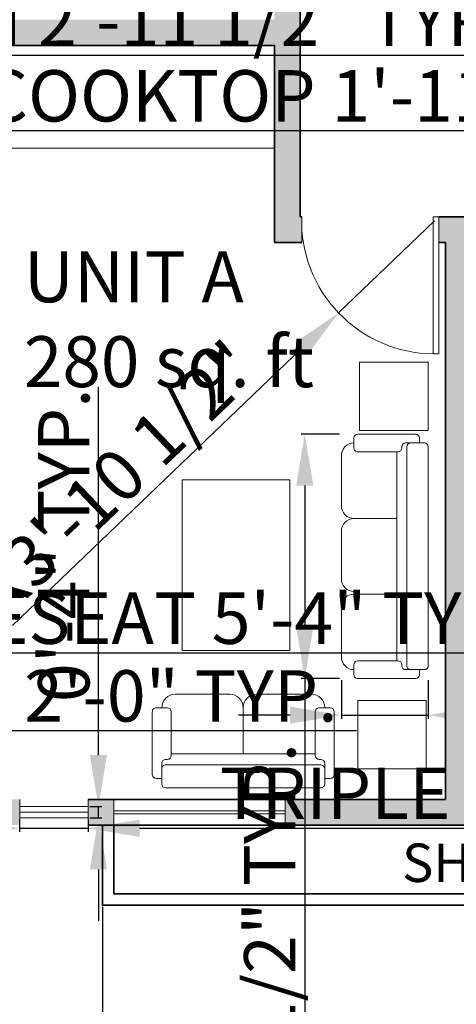
# Model space of a CAD drawing. Units: inches. Extents: x 2043 to 3177, y 1429 to 2563.
# Tile 6 of 14: x 2453 to 2607, y 1608 to 1952. Entities that reach past the tile are written whole.
import ezdxf

# ---------------------------------------------------------------- set-up
doc = ezdxf.new("R2010")
doc.units = ezdxf.units.IN
for name, color, linetype, lineweight in [('A-ANNO-DIMS', 2, 'Continuous', 13), ('A-AREA-IDEN', 7, 'Continuous', 18), ('A-DOOR', 3, 'Continuous', 18), ('A-FLOR-CASE', 8, 'Continuous', 18), ('A-FURN', 8, 'Continuous', 18), ('A-GLAZ', 4, 'Continuous', 18), ('A-WALL', 7, 'Continuous', 35)]:
    doc.layers.add(name, color=color, linetype=linetype, lineweight=lineweight)
doc.layers.add('A-WALL-PATT', color=251, linetype='Continuous', lineweight=13, true_color=0x636466)
doc.styles.get("Standard").update_dxf_attribs({"font": 'arial.ttf'})
doc.dimstyles.new('ISO-25', dxfattribs={"dimtxt": 18, "dimasz": 18, "dimexe": 1.25, "dimexo": 0.625, "dimtad": 1, "dimlunit": 3, "dimtxsty": 'Standard', "dimcen": 2.5, "dimadec": 0, "dimazin": 0, "dimtfac": 1, "dimtmove": 0, "dimatfit": 3, "dimfxl": 1, "dimarcsym": 0})

# ---------------------------------------------------------------- blocks, each defined once
blk = doc.blocks.new('A$C115861F8')
for p, q in [((0.0679, 0.6401), (0.0679, 0.6013)), ((1.7846, 0.6692), (0.097, 0.6692)), ((1.8136, 0.6401), (1.8136, 0.6013)), ((0, 0.5722), (0, 0.1261)), ((0.0679, 0.6013), (0.0291, 0.6013)), ((0.0679, 0.5334), (0.0679, 0.6013)), ((0.0679, 0.4946), (0.0679, 0.5431)), ((1.8136, 0.6013), (1.8524, 0.6013)), ((1.8136, 0.5334), (1.8136, 0.6013)), ((1.8136, 0.4946), (1.8136, 0.5431)), ((1.8815, 0.5722), (1.8815, 0.1261)), ((1.7846, 0.5043), (0.097, 0.5043)), ((0.1067, 0.4655), (0.097, 0.4655)), ((1.7749, 0.4655), (1.7846, 0.4655)), ((0.1358, 0.1261), (0.1358, 0.4364)), ((1.7458, 0.4267), (0.1358, 0.4267)), ((0.6498, 0.097), (0.6498, 0.4267)), ((1.2317, 0.097), (1.2317, 0.4267)), ((1.7458, 0.1261), (1.7458, 0.4364)), ((0.0291, 0.097), (0.1067, 0.097)), ((1.8524, 0.097), (1.7749, 0.097)), ((0.1649, 0), (0.5528, 0)), ((1.1347, 0), (0.7468, 0)), ((1.3287, 0), (1.7167, 0))]:
    blk.add_line(p, q)
for centre, radius, start, end in [((0.097, 0.6401), 0.0291, 90, 180), ((1.7846, 0.6401), 0.0291, 0, 90), ((0.0291, 0.5722), 0.0291, 90, 180), ((0.097, 0.5334), 0.0291, 180, 270), ((1.7846, 0.5334), 0.0291, 270, 0), ((1.8524, 0.5722), 0.0291, 0, 90), ((0.097, 0.4946), 0.0291, 180, 270), ((0.1067, 0.4364), 0.0291, 0, 90), ((1.7749, 0.4364), 0.0291, 90, 180), ((1.7846, 0.4946), 0.0291, 270, 0), ((0.0291, 0.1261), 0.0291, 180, 270), ((0.1649, 0.097), 0.097, 180, 270), ((0.1067, 0.1261), 0.0291, 270, 0), ((0.5528, 0.097), 0.097, 270, 0), ((0.7468, 0.097), 0.097, 180, 270), ((1.1147, 0.097), 0.097, 270, 0), ((1.3287, 0.097), 0.097, 180, 270), ((1.7167, 0.097), 0.097, 270, 0), ((1.7749, 0.1261), 0.0291, 180, 270), ((1.8524, 0.1261), 0.0291, 270, 0)]:
    blk.add_arc(centre, radius, start, end)
blk = doc.blocks.new('A$C02A636C4')
for p, q in [((0.0679, 0.6401), (0.0679, 0.6013)), ((1.2026, 0.6692), (0.097, 0.6692)), ((1.2317, 0.6401), (1.2317, 0.6013)), ((0, 0.5722), (0, 0.1261)), ((0.0679, 0.6013), (0.0291, 0.6013)), ((0.0679, 0.5334), (0.0679, 0.6013)), ((1.2317, 0.6013), (1.2705, 0.6013)), ((1.2317, 0.5334), (1.2317, 0.6013)), ((1.2996, 0.5722), (1.2996, 0.1261)), ((0.0679, 0.4946), (0.0679, 0.5431)), ((1.2026, 0.5043), (0.097, 0.5043)), ((1.2317, 0.4946), (1.2317, 0.5431)), ((0.1067, 0.4655), (0.097, 0.4655)), ((0.1358, 0.1261), (0.1358, 0.4364)), ((1.1638, 0.4267), (0.1358, 0.4267)), ((0.6498, 0.097), (0.6498, 0.4267)), ((1.1638, 0.1261), (1.1638, 0.4364)), ((1.1929, 0.4655), (1.2026, 0.4655)), ((0.0291, 0.097), (0.1067, 0.097)), ((1.2705, 0.097), (1.1929, 0.097)), ((0.1649, 0), (0.5528, 0)), ((0.7468, 0), (1.1347, 0))]:
    blk.add_line(p, q)
for centre, radius, start, end in [((0.097, 0.6401), 0.0291, 90, 180), ((1.2026, 0.6401), 0.0291, 0, 90), ((0.0291, 0.5722), 0.0291, 90, 180), ((1.2705, 0.5722), 0.0291, 0, 90), ((0.097, 0.5334), 0.0291, 180, 270), ((0.097, 0.4946), 0.0291, 180, 270), ((1.2026, 0.5334), 0.0291, 270, 0), ((1.2026, 0.4946), 0.0291, 270, 0), ((0.1067, 0.4364), 0.0291, 0, 90), ((1.1929, 0.4364), 0.0291, 90, 180), ((0.0291, 0.1261), 0.0291, 180, 270), ((0.1649, 0.097), 0.097, 180, 270), ((0.1067, 0.1261), 0.0291, 270, 0), ((0.5528, 0.097), 0.097, 270, 0), ((0.7468, 0.097), 0.097, 180, 270), ((1.1347, 0.097), 0.097, 270, 0), ((1.1929, 0.1261), 0.0291, 180, 270), ((1.2705, 0.1261), 0.0291, 270, 0)]:
    blk.add_arc(centre, radius, start, end)
blk = doc.blocks.new('*D22')
at = {"layer": 'A-ANNO-DIMS', "color": 0, "lineweight": -2, "transparency": 16777216}
for p, q in [((2482.49, 1641.77), (2482.49, 1560.37)), ((2731.99, 1641.77), (2731.99, 1560.37)), ((2500.49, 1561.62), (2713.99, 1561.62))]:
    blk.add_line(p, q, dxfattribs=at)
at = {"layer": 'A-ANNO-DIMS', "color": 0, "transparency": 16777216}
for points in [[(2500.49, 1564.62), (2500.49, 1558.62), (2482.49, 1561.62)], [(2713.99, 1564.62), (2713.99, 1558.62), (2731.99, 1561.62)]]:
    blk.add_solid(points, dxfattribs=at)
at = {"layer": 'Defpoints', "color": 0, "transparency": 16777216}
for p in [(2482.49, 1642.39), (2731.99, 1642.39), (2731.99, 1561.62)]:
    blk.add_point(p, dxfattribs=at)
at = {"layer": 'A-ANNO-DIMS', "color": 0, "transparency": 16777216, "insert": (2607.24, 1571.44), "char_height": 18, "attachment_point": 5}
blk.add_mtext('25\'-0"', dxfattribs=at)
blk = doc.blocks.new('*D23')
at = {"layer": 'A-ANNO-DIMS', "color": 0, "lineweight": -2, "transparency": 16777216}
for p, q in [((2446.74, 1641.77), (2446.74, 1511.06)), ((2482.49, 1641.77), (2482.49, 1511.06)), ((2428.74, 1512.31), (2361.66, 1512.31)), ((2482.49, 1512.31), (2446.74, 1512.31)), ((2500.49, 1512.31), (2518.49, 1512.31))]:
    blk.add_line(p, q, dxfattribs=at)
at = {"layer": 'A-ANNO-DIMS', "color": 0, "transparency": 16777216}
for points in [[(2428.74, 1515.31), (2428.74, 1509.31), (2446.74, 1512.31)], [(2500.49, 1515.31), (2500.49, 1509.31), (2482.49, 1512.31)]]:
    blk.add_solid(points, dxfattribs=at)
at = {"layer": 'Defpoints', "color": 0, "transparency": 16777216}
for p in [(2446.74, 1642.39), (2482.49, 1642.39), (2446.74, 1512.31)]:
    blk.add_point(p, dxfattribs=at)
at = {"layer": 'A-ANNO-DIMS', "color": 0, "transparency": 16777216, "insert": (2386.2, 1522.13), "char_height": 18, "attachment_point": 5}
blk.add_mtext('3\'-0"', dxfattribs=at)
blk = doc.blocks.new('*D29')
at = {"layer": 'A-ANNO-DIMS', "color": 0, "lineweight": -2, "transparency": 16777216}
for p, q in [((2233.74, 1633.77), (2233.74, 1430.58)), ((2980.74, 1633.77), (2980.74, 1430.58)), ((2251.74, 1431.83), (2962.74, 1431.83))]:
    blk.add_line(p, q, dxfattribs=at)
at = {"layer": 'A-ANNO-DIMS', "color": 0, "transparency": 16777216}
for points in [[(2251.74, 1434.83), (2251.74, 1428.83), (2233.74, 1431.83)], [(2962.74, 1434.83), (2962.74, 1428.83), (2980.74, 1431.83)]]:
    blk.add_solid(points, dxfattribs=at)
at = {"layer": 'Defpoints', "color": 0, "transparency": 16777216}
for p in [(2233.74, 1634.39), (2980.74, 1634.39), (2980.74, 1431.83)]:
    blk.add_point(p, dxfattribs=at)
at = {"layer": 'A-ANNO-DIMS', "color": 0, "transparency": 16777216, "insert": (2607.24, 1441.64), "char_height": 18, "attachment_point": 5}
blk.add_mtext('75\'-0"', dxfattribs=at)
blk = doc.blocks.new('END-TABLE-24')
blk.add_lwpolyline([(24, 24), (24, 0), (0, 0), (0, 24)], close=True)
blk = doc.blocks.new('COFFEE-TABLE-RECT')
blk.add_lwpolyline([(0, 59.71), (37.81, 59.71), (37.81, 0), (0, 0)], close=True)
blk = doc.blocks.new('GLAZING-24-TRIPLE')
for p, q in [((24, 4), (0, 4)), ((24, 2), (0, 2)), ((24, 0), (0, 0))]:
    blk.add_line(p, q)
blk = doc.blocks.new('GLAZING-60')
for p, q in [((0, 1), (60, 1)), ((0, 0), (60, 0))]:
    blk.add_line(p, q)
blk = doc.blocks.new('*D43')
at = {"layer": 'A-ANNO-DIMS', "color": 0, "lineweight": -2, "transparency": 16777216}
for p, q in [((2565.6, 1807.28), (2552.15, 1807.28)), ((2553.4, 1789.28), (2553.4, 1739.74)), ((2565.6, 1721.74), (2552.15, 1721.74)), ((2553.4, 1721.74), (2553.4, 1475.47))]:
    blk.add_line(p, q, dxfattribs=at)
at = {"layer": 'A-ANNO-DIMS', "color": 0, "transparency": 16777216}
for points in [[(2550.4, 1789.28), (2556.4, 1789.28), (2553.4, 1807.28)], [(2550.4, 1739.74), (2556.4, 1739.74), (2553.4, 1721.74)]]:
    blk.add_solid(points, dxfattribs=at)
at = {"layer": 'Defpoints', "color": 0, "transparency": 16777216}
for p in [(2566.23, 1807.28), (2553.4, 1721.74), (2566.23, 1721.74)]:
    blk.add_point(p, dxfattribs=at)
at = {"layer": 'A-ANNO-DIMS', "color": 0, "transparency": 16777216, "insert": (2543.46, 1589.61), "char_height": 18, "attachment_point": 5, "rotation": 90}
blk.add_mtext('SOFA 7\'-1 1/2" TYP.', dxfattribs=at)
blk = doc.blocks.new('*D44')
at = {"layer": 'A-ANNO-DIMS', "color": 0, "lineweight": -2, "transparency": 16777216}
for p, q in [((2566.23, 1721.12), (2566.23, 1707.66)), ((2596.65, 1721.12), (2596.65, 1707.66)), ((2548.23, 1708.91), (2530.23, 1708.91)), ((2566.23, 1708.91), (2596.65, 1708.91)), ((2614.65, 1708.91), (2785.87, 1708.91))]:
    blk.add_line(p, q, dxfattribs=at)
at = {"layer": 'A-ANNO-DIMS', "color": 0, "transparency": 16777216}
for points in [[(2548.23, 1711.91), (2548.23, 1705.91), (2566.23, 1708.91)], [(2614.65, 1711.91), (2614.65, 1705.91), (2596.65, 1708.91)]]:
    blk.add_solid(points, dxfattribs=at)
at = {"layer": 'Defpoints', "color": 0, "transparency": 16777216}
for p in [(2566.23, 1721.74), (2596.65, 1721.74), (2596.65, 1708.91)]:
    blk.add_point(p, dxfattribs=at)
at = {"layer": 'A-ANNO-DIMS', "color": 0, "transparency": 16777216, "insert": (2709.26, 1718.85), "char_height": 18, "attachment_point": 5}
blk.add_mtext('2\'-6 1/2" TYP.', dxfattribs=at)
blk = doc.blocks.new('*D45')
at = {"layer": 'A-ANNO-DIMS', "color": 0, "lineweight": -2, "transparency": 16777216}
for p, q in [((2656.49, 1721.63), (2656.49, 1731.82)), ((2720.27, 1721.63), (2720.27, 1731.82)), ((2656.49, 1730.57), (2388.57, 1730.57)), ((2702.27, 1730.57), (2674.49, 1730.57))]:
    blk.add_line(p, q, dxfattribs=at)
at = {"layer": 'A-ANNO-DIMS', "color": 0, "transparency": 16777216}
for points in [[(2674.49, 1733.57), (2674.49, 1727.57), (2656.49, 1730.57)], [(2702.27, 1733.57), (2702.27, 1727.57), (2720.27, 1730.57)]]:
    blk.add_solid(points, dxfattribs=at)
at = {"layer": 'Defpoints', "color": 0, "transparency": 16777216}
for p in [(2656.49, 1730.57), (2656.49, 1721), (2720.27, 1721)]:
    blk.add_point(p, dxfattribs=at)
at = {"layer": 'A-ANNO-DIMS', "color": 0, "transparency": 16777216, "insert": (2513.53, 1740.51), "char_height": 18, "attachment_point": 5}
blk.add_mtext('LOVESEAT 5\'-4" TYP.', dxfattribs=at)
blk = doc.blocks.new('*D47')
at = {"layer": 'A-ANNO-DIMS', "color": 0, "lineweight": -2, "transparency": 16777216}
for p, q in [((2236.77, 1703.49), (2218.77, 1703.49)), ((2254.77, 1700.52), (2254.77, 1704.74)), ((2254.77, 1703.49), (2278.77, 1703.49)), ((2278.77, 1700.52), (2278.77, 1704.74)), ((2296.77, 1703.49), (2571.52, 1703.49))]:
    blk.add_line(p, q, dxfattribs=at)
at = {"layer": 'A-ANNO-DIMS', "color": 0, "transparency": 16777216}
for points in [[(2236.77, 1706.49), (2236.77, 1700.49), (2254.77, 1703.49)], [(2296.77, 1706.49), (2296.77, 1700.49), (2278.77, 1703.49)]]:
    blk.add_solid(points, dxfattribs=at)
at = {"layer": 'Defpoints', "color": 0, "transparency": 16777216}
for p in [(2278.77, 1703.49), (2254.77, 1699.89), (2278.77, 1699.89)]:
    blk.add_point(p, dxfattribs=at)
at = {"layer": 'A-ANNO-DIMS', "color": 0, "transparency": 16777216, "insert": (2443.14, 1713.31), "char_height": 18, "attachment_point": 5}
blk.add_mtext('END TABLE 2\'-0" TYP.', dxfattribs=at)
blk = doc.blocks.new('*D57')
at = {"layer": 'A-ANNO-DIMS', "color": 0, "lineweight": -2, "transparency": 16777216}
for p, q in [((2309.03, 1935.24), (2309.03, 1941.18)), ((2344.46, 1935.24), (2344.46, 1941.18)), ((2291.03, 1939.93), (2273.03, 1939.93)), ((2309.03, 1939.93), (2344.46, 1939.93)), ((2362.46, 1939.93), (2629.01, 1939.93))]:
    blk.add_line(p, q, dxfattribs=at)
at = {"layer": 'A-ANNO-DIMS', "color": 0, "transparency": 16777216}
for points in [[(2291.03, 1942.93), (2291.03, 1936.93), (2309.03, 1939.93)], [(2362.46, 1942.93), (2362.46, 1936.93), (2344.46, 1939.93)]]:
    blk.add_solid(points, dxfattribs=at)
at = {"layer": 'Defpoints', "color": 0, "transparency": 16777216}
for p in [(2344.46, 1939.93), (2309.03, 1934.62), (2344.46, 1934.62)]:
    blk.add_point(p, dxfattribs=at)
at = {"layer": 'A-ANNO-DIMS', "color": 0, "transparency": 16777216, "insert": (2504.74, 1949.86), "char_height": 18, "attachment_point": 5}
blk.add_mtext('BASIN 2\'-11 1/2" TYP.', dxfattribs=at)
blk = doc.blocks.new('*D61')
at = {"layer": 'A-ANNO-DIMS', "color": 0, "lineweight": -2, "transparency": 16777216}
for p, q in [((2752.39, 1913.46), (2434.98, 1913.46)), ((2770.39, 1916.38), (2770.39, 1912.21)), ((2794.01, 1913.46), (2770.39, 1913.46)), ((2794.01, 1916.38), (2794.01, 1912.21)), ((2812.01, 1913.46), (2830.01, 1913.46))]:
    blk.add_line(p, q, dxfattribs=at)
at = {"layer": 'A-ANNO-DIMS', "color": 0, "transparency": 16777216}
for points in [[(2752.39, 1916.46), (2752.39, 1910.46), (2770.39, 1913.46)], [(2812.01, 1916.46), (2812.01, 1910.46), (2794.01, 1913.46)]]:
    blk.add_solid(points, dxfattribs=at)
at = {"layer": 'Defpoints', "color": 0, "transparency": 16777216}
for p in [(2770.39, 1917.01), (2794.01, 1917.01), (2770.39, 1913.46)]:
    blk.add_point(p, dxfattribs=at)
at = {"layer": 'A-ANNO-DIMS', "color": 0, "transparency": 16777216, "insert": (2584.68, 1923.4), "char_height": 18, "attachment_point": 5}
blk.add_mtext('COOKTOP 1\'-11 1/2" TYP.', dxfattribs=at)
blk = doc.blocks.new('*D67')
at = {"layer": 'A-ANNO-DIMS', "color": 0, "lineweight": -2, "transparency": 16777216}
for p, q in [((2453.49, 1672.27), (2453.49, 1668.04)), ((2477.49, 1672.27), (2477.49, 1668.04)), ((2435.49, 1669.29), (2417.49, 1669.29)), ((2453.49, 1669.29), (2477.49, 1669.29)), ((2495.49, 1669.29), (2837.31, 1669.29))]:
    blk.add_line(p, q, dxfattribs=at)
at = {"layer": 'A-ANNO-DIMS', "color": 0, "transparency": 16777216}
for points in [[(2435.49, 1672.29), (2435.49, 1666.29), (2453.49, 1669.29)], [(2495.49, 1672.29), (2495.49, 1666.29), (2477.49, 1669.29)]]:
    blk.add_solid(points, dxfattribs=at)
at = {"layer": 'Defpoints', "color": 0, "transparency": 16777216}
for p in [(2453.49, 1672.89), (2477.49, 1672.89), (2477.49, 1669.29)]:
    blk.add_point(p, dxfattribs=at)
at = {"layer": 'A-ANNO-DIMS', "color": 0, "transparency": 16777216, "insert": (2675.4, 1679.23), "char_height": 18, "attachment_point": 5}
blk.add_mtext('TRIPLE GLAZING 2\'-0" TYP.', dxfattribs=at)
blk = doc.blocks.new('*D68')
at = {"layer": 'A-ANNO-DIMS', "color": 0, "lineweight": -2, "transparency": 16777216}
for p, q in [((2481.09, 1694.89), (2481.09, 1823.86)), ((2478.12, 1676.89), (2482.34, 1676.89)), ((2481.09, 1672.89), (2481.09, 1676.89)), ((2478.12, 1672.89), (2482.34, 1672.89)), ((2481.09, 1654.89), (2481.09, 1636.89))]:
    blk.add_line(p, q, dxfattribs=at)
at = {"layer": 'A-ANNO-DIMS', "color": 0, "transparency": 16777216}
for points in [[(2478.09, 1694.89), (2484.09, 1694.89), (2481.09, 1676.89)], [(2478.09, 1654.89), (2484.09, 1654.89), (2481.09, 1672.89)]]:
    blk.add_solid(points, dxfattribs=at)
at = {"layer": 'Defpoints', "color": 0, "transparency": 16777216}
for p in [(2477.49, 1676.89), (2481.09, 1676.89), (2477.49, 1672.89)]:
    blk.add_point(p, dxfattribs=at)
at = {"layer": 'A-ANNO-DIMS', "color": 0, "transparency": 16777216, "insert": (2471.28, 1768.38), "char_height": 18, "attachment_point": 5, "rotation": 90}
blk.add_mtext('0\'-4" TYP.', dxfattribs=at)
blk = doc.blocks.new('*D86')
at = {"layer": 'A-ANNO-DIMS', "color": 0, "lineweight": -2, "transparency": 16777216}
for p, q in [((2598.87, 1881.94), (2565.26, 1849.73)), ((2451, 1740.24), (2552.26, 1837.28))]:
    blk.add_line(p, q, dxfattribs=at)
at = {"layer": 'A-ANNO-DIMS', "color": 0, "transparency": 16777216}
blk.add_solid([(2550.18, 1839.44), (2554.34, 1835.11), (2565.26, 1849.73)], dxfattribs=at)
at = {"layer": 'Defpoints', "color": 0, "transparency": 16777216}
for p in [(2598.87, 1881.94), (2565.26, 1849.73)]:
    blk.add_point(p, dxfattribs=at)
at = {"layer": 'A-ANNO-DIMS', "color": 0, "transparency": 16777216, "insert": (2488.26, 1789.71), "char_height": 18, "attachment_point": 5, "rotation": 43.781}
blk.add_mtext('R3\'-10 1/2"', dxfattribs=at)

msp = doc.modelspace()

# ---------------------------------------------------------------- hatches: boundary and pattern name
at = {"layer": 'A-WALL-PATT'}
h = msp.add_hatch(color=256, dxfattribs=at)
h.dxf.hatch_style = 1
h.paths.add_polyline_path([(2283.62, 2261.393), (2233.745, 2261.393), (2233.745, 2029.268), (2242.745, 2029.268), (2242.745, 2070.143), (2348.495, 2070.143), (2348.495, 2063.887), (2352.995, 2063.887), (2352.995, 2094.143), (2353.364, 2094.143, -0.017175), (2353.364, 2096.932), (2353.364, 2098.643), (2348.495, 2098.643), (2348.495, 2096.393), (2348.495, 2074.643), (2242.745, 2074.643), (2242.745, 2252.393), (2283.62, 2252.393)])
h.paths.add_polyline_path([(2453.87, 2261.393), (2355.62, 2261.393), (2355.62, 2252.393), (2396.495, 2252.393), (2396.495, 2098.643), (2395.364, 2098.643), (2395.364, 2094.143), (2436.995, 2094.143), (2436.995, 2098.643), (2400.995, 2098.643), (2400.995, 2252.393), (2453.87, 2252.393)])
h.paths.add_polyline_path([(2551.745, 2261.393), (2489.87, 2261.393), (2489.87, 2252.393), (2542.745, 2252.393), (2542.745, 2098.643), (2506.745, 2098.643), (2506.745, 2094.143), (2542.745, 2094.143), (2542.745, 2003.513), (2549.809, 2003.513, -0.0102854), (2551.745, 2003.513), (2551.745, 2195.393), (2571.245, 2195.393), (2571.245, 2204.393), (2551.745, 2204.393)])
h.paths.add_polyline_path([(2724.62, 2261.393), (2662.745, 2261.393), (2662.745, 2204.393), (2643.245, 2204.393), (2643.245, 2195.393), (2662.745, 2195.393), (2662.745, 2002.566, -0.0156152), (2665.651, 2002.566), (2671.745, 2002.566), (2671.745, 2094.143), (2707.745, 2094.143), (2707.745, 2098.643), (2671.745, 2098.643), (2671.745, 2252.393), (2724.62, 2252.393)])
h.paths.add_polyline_path([(2858.87, 2261.393), (2760.62, 2261.393), (2760.62, 2252.393), (2813.495, 2252.393), (2813.495, 2098.643), (2777.495, 2098.643), (2777.495, 2094.143), (2819.302, 2094.143), (2819.302, 2098.643), (2817.995, 2098.643), (2817.995, 2252.393), (2858.87, 2252.393)])
h.paths.add_polyline_path([(2980.745, 2261.393), (2930.87, 2261.393), (2930.87, 2252.393), (2971.745, 2252.393), (2971.745, 2074.643), (2865.995, 2074.643), (2865.995, 2098.643), (2861.429, 2098.643, -0.0279128), (2861.495, 2094.143), (2861.495, 2063.254), (2865.995, 2063.254), (2865.995, 2070.143), (2971.745, 2070.143), (2971.745, 2029.268), (2980.745, 2029.268)])
h.paths.add_polyline_path([(2980.745, 1993.268), (2971.745, 1993.268), (2971.745, 1952.393), (2865.995, 1952.393), (2865.995, 2027.254), (2865.688, 2027.254, -0.0309542), (2861.495, 2027.254), (2861.495, 1952.393), (2671.745, 1952.393), (2671.745, 1954.566), (2662.745, 1954.566), (2662.745, 1883.393), (2661.473, 1883.393, -0.012912), (2661.473, 1880.977), (2661.473, 1874.393), (2671.745, 1874.393), (2671.745, 1943.393), (2861.495, 1943.393), (2861.495, 1903.412, -0.0351753), (2865.995, 1903.659), (2865.995, 1943.393), (2971.745, 1943.393), (2971.745, 1922.018), (2980.745, 1922.018)])
h.paths.add_polyline_path([(2980.745, 1886.018), (2971.745, 1886.018), (2971.745, 1864.643), (2865.995, 1864.643), (2865.995, 1867.412), (2861.495, 1867.412), (2861.495, 1840.643), (2828.844, 1840.643, -0.0159075), (2828.844, 1837.684), (2828.844, 1836.143), (2865.995, 1836.143), (2865.995, 1860.143), (2971.745, 1860.143), (2971.745, 1643.393), (2910.245, 1643.393), (2910.245, 1634.393), (2980.745, 1634.393)])
h.paths.add_polyline_path([(2776.745, 1836.143), (2780.844, 1836.143), (2780.844, 1840.643), (2772.245, 1840.643), (2772.245, 1679.393), (2760.995, 1679.393), (2760.995, 1670.393), (2767.745, 1670.393), (2767.745, 1634.393), (2838.245, 1634.393), (2838.245, 1643.393), (2776.745, 1643.393)])
h.paths.add_polyline_path([(2736.995, 1679.393), (2727.995, 1679.393), (2727.995, 1670.393), (2736.995, 1670.393)])
h.paths.add_polyline_path([(2667.995, 1679.393), (2611.745, 1679.393), (2611.745, 1874.393), (2613.473, 1874.393), (2613.473, 1883.393), (2600.336, 1883.393), (2600.336, 1874.393), (2602.745, 1874.393), (2602.745, 1679.393), (2546.495, 1679.393), (2546.495, 1670.393), (2667.995, 1670.393)])
h.paths.add_polyline_path([(2486.495, 1679.393), (2477.495, 1679.393), (2477.495, 1670.393), (2486.495, 1670.393)])
h.paths.add_polyline_path([(2453.495, 1679.393), (2442.245, 1679.393), (2442.245, 1839.893), (2427.654, 1839.893), (2427.654, 1835.393), (2437.745, 1835.393), (2437.745, 1643.393), (2376.245, 1643.393), (2376.245, 1634.393), (2446.745, 1634.393), (2446.745, 1670.393), (2453.495, 1670.393)])
h.paths.add_polyline_path([(2304.245, 1643.393), (2242.745, 1643.393), (2242.745, 1857.143), (2348.495, 1857.143), (2348.495, 1835.393), (2352.995, 1835.393), (2379.654, 1835.393), (2379.654, 1837.073, -0.0151369), (2379.654, 1839.893), (2352.995, 1839.893), (2352.995, 1867.394), (2348.495, 1867.394), (2348.495, 1861.643), (2242.745, 1861.643), (2242.745, 1884.518), (2233.745, 1884.518), (2233.745, 1634.393), (2304.245, 1634.393)])
h.paths.add_polyline_path([(2551.745, 1955.513), (2542.745, 1955.513), (2542.745, 1952.393), (2352.995, 1952.393), (2352.995, 2027.887, -0.0208198), (2350.117, 2027.887), (2348.495, 2027.887), (2348.495, 1952.393), (2242.745, 1952.393), (2242.745, 1993.268), (2233.745, 1993.268), (2233.745, 1943.393), (2233.745, 1920.518), (2242.745, 1920.518), (2242.745, 1943.393), (2348.495, 1943.393), (2348.495, 1903.394), (2352.995, 1903.394), (2352.995, 1943.393), (2542.745, 1943.393), (2542.745, 1874.393), (2552.336, 1874.393), (2552.336, 1880.494, -0.0155728), (2552.336, 1883.393), (2551.745, 1883.393)])

# ---------------------------------------------------------------- linework, layer by layer
at = {"layer": 'A-DOOR'}
for p, q in [((2552.336, 1883.393), (2552.336, 1874.393)), ((2598.336, 1835.393), (2598.336, 1883.393)), ((2598.336, 1883.393), (2600.336, 1883.393)), ((2600.336, 1883.393), (2600.336, 1874.393)), ((2600.336, 1883.393), (2600.336, 1835.393)), ((2600.336, 1835.393), (2598.336, 1835.393))]:
    msp.add_line(p, q, dxfattribs=at)
msp.add_arc((2598.867, 1881.944), 46.553, 178.21564, 269.34661, dxfattribs=at)
at = {"layer": 'A-FLOR-CASE'}
msp.add_line((2352.995, 1907.393), (2542.745, 1907.393), dxfattribs=at)
at = {"layer": 'A-GLAZ'}
for p, q in [((2453.495, 1679.393), (2453.495, 1670.393)), ((2477.495, 1679.393), (2477.495, 1670.393)), ((2486.495, 1679.393), (2486.495, 1670.393)), ((2546.495, 1679.393), (2546.495, 1670.393))]:
    msp.add_line(p, q, dxfattribs=at)
at = {"layer": 'A-WALL'}
for p, q in [((2551.745, 1955.513), (2551.745, 1883.393)), ((2352.995, 1943.393), (2542.745, 1943.393)), ((2542.745, 1943.393), (2542.745, 1874.393)), ((2551.745, 1883.393), (2552.336, 1883.393)), ((2600.336, 1883.393), (2613.473, 1883.393)), ((2542.745, 1874.393), (2552.336, 1874.393)), ((2600.336, 1874.393), (2602.745, 1874.393)), ((2602.745, 1679.393), (2602.745, 1874.393)), ((2477.495, 1679.393), (2602.745, 1679.393)), ((2477.495, 1670.393), (2736.995, 1670.393)), ((2482.495, 1670.393), (2482.495, 1642.393)), ((2486.495, 1670.393), (2486.495, 1646.393)), ((2486.495, 1646.393), (2727.995, 1646.393)), ((2482.495, 1642.393), (2731.995, 1642.393))]:
    msp.add_line(p, q, dxfattribs=at)

# ---------------------------------------------------------------- block references
at = {"layer": 'A-FURN'}
for name, p in [('END-TABLE-24', (2572.618, 1808.509)), ('COFFEE-TABLE-RECT', (2510.409, 1731.521)), ('END-TABLE-24', (2571.99, 1690.066))]:
    msp.add_blockref(name, p, dxfattribs=at)
for name, p, xscale, yscale, zscale, rotation in [('A$C115861F8', (2566.23, 1807.279), 45.45990975277036, 45.45990975277036, 45.45990975277036, 270), ('A$C02A636C4', (2563.737, 1716.244), 49.07597789630211, 49.07597789630211, 49.07597789630211, 180)]:
    msp.add_blockref(name, p, dxfattribs=dict(at, xscale=xscale, yscale=yscale, zscale=zscale, rotation=rotation))
at = {"layer": 'A-GLAZ'}
for name, p in [('GLAZING-24-TRIPLE', (2453.495, 1672.893)), ('GLAZING-60', (2486.495, 1674.393))]:
    msp.add_blockref(name, p, dxfattribs=at)

# ---------------------------------------------------------------- texts
at = {"layer": 'A-AREA-IDEN', "attachment_point": 1}
for s, width, gutter_width, insert, char_height in [('UNIT A \\P280 sq. ft', 505.18079, 89.135, (2454.954, 1871.29), 17.8269), ('SHAFT', 381.44992, 67.303, (2587.501, 1663.948), 13.4607)]:
    msp.add_mtext_dynamic_manual_height_columns(s, width=width, gutter_width=gutter_width, heights=[0], dxfattribs=dict(at, insert=insert, char_height=char_height))

# ---------------------------------------------------------------- dimensions: what is measured, and where the dimension line sits
at = {"layer": 'A-ANNO-DIMS'}
for base, p1, p2, text, override, picture, middle in [((2344.462, 1939.932), (2309.031, 1934.617), (2344.462, 1934.617), 'BASIN <> TYP.', {"dimdec": 1, "dimlfac": 1, "dimrnd": 0, "dimzin": 1, "dimdsep": 46, "dimlunit": 4, "dimfrac": 2}, '*D57', (2504.735, 1949.864)), ((2278.767, 1703.49), (2254.767, 1699.89), (2278.767, 1699.89), 'END TABLE <> TYP.', {"dimdec": 1, "dimlfac": 1, "dimrnd": 0, "dimzin": 1, "dimdsep": 46, "dimlunit": 4, "dimfrac": 2}, '*D47', (2443.142, 1713.306)), ((2596.652, 1708.915), (2566.23, 1721.745), (2596.652, 1721.745), '<> TYP.', {"dimdec": 1, "dimlfac": 1, "dimrnd": 0, "dimzin": 1, "dimdsep": 46, "dimlunit": 4, "dimfrac": 2}, '*D44', (2709.261, 1718.847)), ((2477.495, 1669.293), (2453.495, 1672.893), (2477.495, 1672.893), 'TRIPLE GLAZING <> TYP.', {"dimdec": 1, "dimlfac": 1, "dimrnd": 0, "dimzin": 1, "dimdsep": 46, "dimlunit": 4, "dimfrac": 2}, '*D67', (2675.401, 1679.225)), ((2446.745, 1512.311), (2482.495, 1642.393), (2446.745, 1642.393), '3\'-0"', {"dimclrd": 0, "dimclre": 0, "dimclrt": 0}, '*D23', (2386.201, 1522.132)), ((2731.995, 1561.62), (2482.495, 1642.393), (2731.995, 1642.393), '25\'-0"', {"dimclrd": 0, "dimclre": 0, "dimclrt": 0}, '*D22', (2607.245, 1571.436)), ((2980.745, 1431.826), (2233.745, 1634.393), (2980.745, 1634.393), '75\'-0"', {"dimclrd": 0, "dimclre": 0, "dimclrt": 0}, '*D29', (2607.245, 1441.642))]:
    dim = msp.add_linear_dim(base=base, p1=p1, p2=p2, text=text, dimstyle='ISO-25', override=override, dxfattribs=at)
    dim.commit()
    dim.dimension.update_dxf_attribs({"geometry": picture, "text_midpoint": middle})
for base, p1, p2, angle, text, picture, middle in [((2770.393, 1913.464), (2794.015, 1917.007), (2770.393, 1917.007), 180, 'COOKTOP <> TYP.', '*D61', (2584.685, 1923.402)), ((2481.095, 1676.893), (2477.495, 1672.893), (2477.495, 1676.893), 90, '<> TYP.', '*D68', (2471.279, 1768.378)), ((2553.4, 1721.745), (2566.23, 1807.279), (2566.23, 1721.745), 270, 'SOFA <> TYP.', '*D43', (2543.461, 1589.607)), ((2656.494, 1730.571), (2720.274, 1721.004), (2656.494, 1721.004), 180, 'LOVESEAT <> TYP.', '*D45', (2513.532, 1740.509))]:
    dim = msp.add_linear_dim(base=base, p1=p1, p2=p2, angle=angle, text=text, dimstyle='ISO-25', override={"dimdec": 1, "dimlfac": 1, "dimrnd": 0, "dimzin": 1, "dimdsep": 46, "dimlunit": 4, "dimfrac": 2}, dxfattribs=at)
    dim.commit()
    dim.dimension.update_dxf_attribs({"geometry": picture, "text_midpoint": middle})
dim = msp.add_radius_dim(center=(2598.867, 1881.944), mpoint=(2565.256, 1849.733), dimstyle='ISO-25', override={"dimdec": 1, "dimlfac": 1, "dimrnd": 0, "dimzin": 1, "dimdsep": 46, "dimlunit": 4, "dimfrac": 2}, dxfattribs=at)
dim.commit()
dim.dimension.update_dxf_attribs({"geometry": '*D86', "text_midpoint": (2488.256, 1789.706)})

doc.saveas('drawing.dxf')
